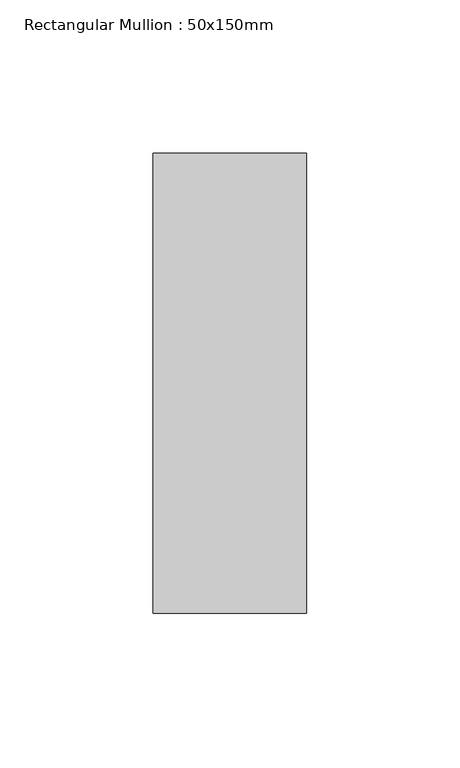
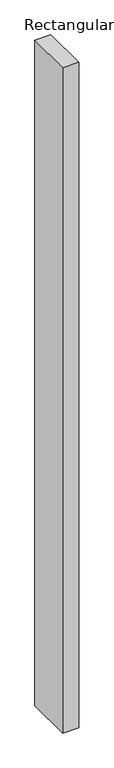
"""IFC4 building model written with IfcOpenShell, lengths in millimetres: member geometry, Rectangular Mullion : 50x150mm."""

from ifc_helpers import new_model, si_unit, frame, origin, place, context, project, spatial, polyline, outline, extrude, source, transform, mapped, element, save


def rectangular_mullion_50x150mm_7233a1e1(model_context):
    return source(origin(), model_context, "Body", "SweptSolid", [
        extrude(outline(polyline([(0.0, 75.0), (0.0, -75.0), (-50.0, -75.0), (-50.0, 75.0), (0.0, 75.0)])), frame((0.0, 0.0, -2196.7065107), z_axis=(0.0, 0.0, 1.0), x_axis=(1.0, 0.0, 0.0)), (0.0, 0.0, 1.0), 2196.7065107),
    ])


if __name__ == "__main__":
    model = new_model("IFC4")
    model_context = context("Model", 3, world=origin())
    ifc_project = project(units=[si_unit("LENGTHUNIT", "METRE", prefix="MILLI")], contexts=[model_context])
    site = spatial("IfcSite", under=ifc_project)
    building = spatial("IfcBuilding", under=site)
    placement = place(None, origin())
    rectangular_mullion_50x150mm_shape = rectangular_mullion_50x150mm_7233a1e1(model_context)
    element("IfcMember", 1, ObjectType="Rectangular Mullion : 50x150mm", at=placement, inside=building, context=model_context, shape_type="MappedRepresentation", body=[
        mapped(rectangular_mullion_50x150mm_shape, transform((0.0, 0.0, 0.0), x_axis=(1.0, 0.0, 0.0), y_axis=(0.0, 1.0, 0.0), z_axis=(0.0, 0.0, 1.0))),
    ])
    save(model, "model.ifc")

# Revit data of these elements
# Type "Rectangular Mullion : 50x150mm"
#   Keynote = "H11"
#   built-in parameter 1007304 = 0.492126 (stored number, unit not read)
#   built-in parameter 1007301 = 0.082021 (stored number, unit not read)
#   built-in parameter 1007300 = 0.082021 (stored number, unit not read)
# Element 1 (IfcMember, "Rectangular Mullion : 50x150mm")
#   Materials on its faces: "Aluminium"
# Materials
#   "Aluminium": class "Metal", colour RGB 247 247 247, transparency 0, Description = "Aluminium 6061", Cost = 0
